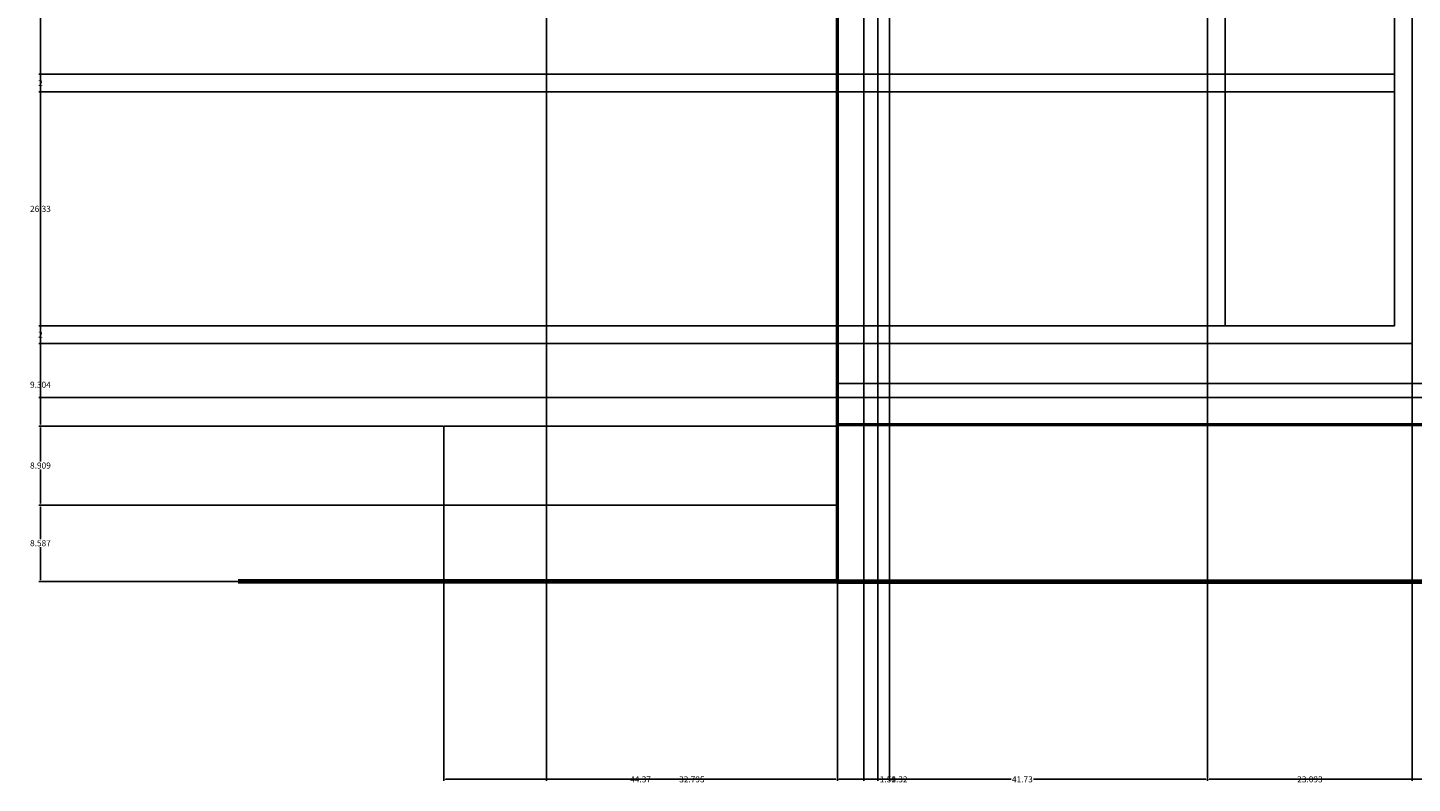
# Model space of a CAD drawing. Units: inches. Extents: x -139 to 346, y 72 to 413.
# Tile 1 of 18: x -139 to 18, y 72 to 157. Entities that reach past the tile are written whole.
import ezdxf

# ---------------------------------------------------------------- set-up
doc = ezdxf.new("R2010")
doc.units = ezdxf.units.IN
doc.header["$MEASUREMENT"] = 0
for name, color, linetype, lineweight in [('A-ANNO-DIMS', 2, 'Continuous', 18), ('A-FLOR-STRS', 2, 'Continuous', 25), ('A-GLAZ', 4, 'Continuous', 25), ('A-WALL', 7, 'Continuous', 50), ('C-TOPO', 7, 'Continuous', 70)]:
    doc.layers.add(name, color=color, linetype=linetype, lineweight=lineweight)
doc.styles.get("Standard").update_dxf_attribs({"font": 'arial.ttf'})
doc.dimstyles.get("Standard").update_dxf_attribs({"dimtxt": 0.6875, "dimasz": 0.18, "dimexe": 0.18, "dimexo": 0.0625, "dimgap": 0.09, "dimtad": 0, "dimtih": 1, "dimtoh": 1, "dimdec": 4, "dimzin": 0, "dimdsep": 46, "dimlunit": 4, "dimtxsty": 'Standard', "dimcen": 0.09, "dimadec": 0, "dimazin": 0, "dimtfac": 1, "dimtdec": 4, "dimtofl": 0, "dimtmove": 0, "dimatfit": 3, "dimfxl": 1, "dimtolj": 1, "dimtzin": 0, "dimarcsym": 0})

# ---------------------------------------------------------------- blocks, each defined once
blk = doc.blocks.new('*D7')
at = {"layer": 'A-ANNO-DIMS', "color": 0, "lineweight": -2, "transparency": 16777216}
for p, q in [((-47.27, 95.04), (-47.27, 117.45)), ((-47.09, 117.27), (129.79, 117.27)), ((309.71, 117.27), (132.82, 117.27)), ((309.89, 95.04), (309.89, 117.45))]:
    blk.add_line(p, q, dxfattribs=at)
at = {"layer": 'A-ANNO-DIMS', "color": 0, "transparency": 16777216}
for points in [[(-47.09, 117.3), (-47.09, 117.24), (-47.27, 117.27)], [(309.71, 117.3), (309.71, 117.24), (309.89, 117.27)]]:
    blk.add_solid(points, dxfattribs=at)
at = {"layer": 'Defpoints', "color": 0, "transparency": 16777216}
for p in [(309.89, 117.27), (-47.27, 94.97), (309.89, 94.97)]:
    blk.add_point(p, dxfattribs=at)
at = {"layer": 'A-ANNO-DIMS', "color": 0, "transparency": 16777216, "insert": (131.31, 117.27), "char_height": 0.688, "attachment_point": 5}
blk.add_mtext('\\A1;357.16', dxfattribs=at)
blk = doc.blocks.new('*D8')
at = {"layer": 'A-ANNO-DIMS', "color": 0, "lineweight": -2, "transparency": 16777216}
for p, q in [((-91.64, 94.91), (-91.64, 72.49)), ((-47.27, 94.91), (-47.27, 72.49)), ((-91.46, 72.67), (-70.72, 72.67)), ((-47.45, 72.67), (-68.19, 72.67))]:
    blk.add_line(p, q, dxfattribs=at)
at = {"layer": 'A-ANNO-DIMS', "color": 0, "transparency": 16777216}
for points in [[(-91.46, 72.7), (-91.46, 72.64), (-91.64, 72.67)], [(-47.45, 72.7), (-47.45, 72.64), (-47.27, 72.67)]]:
    blk.add_solid(points, dxfattribs=at)
at = {"layer": 'Defpoints', "color": 0, "transparency": 16777216}
for p in [(-91.64, 94.97), (-47.27, 94.97), (-47.27, 72.67)]:
    blk.add_point(p, dxfattribs=at)
at = {"layer": 'A-ANNO-DIMS', "color": 0, "transparency": 16777216, "insert": (-69.46, 72.67), "char_height": 0.688, "attachment_point": 5}
blk.add_mtext('\\A1;44.37', dxfattribs=at)
blk = doc.blocks.new('*D9')
at = {"layer": 'A-ANNO-DIMS', "color": 0, "lineweight": -2, "transparency": 16777216}
for p, q in [((-5.54, 121.71), (-5.54, 72.49)), ((-47.27, 112.54), (-47.27, 72.49)), ((-47.09, 72.67), (-27.67, 72.67)), ((-5.72, 72.67), (-25.14, 72.67))]:
    blk.add_line(p, q, dxfattribs=at)
at = {"layer": 'A-ANNO-DIMS', "color": 0, "transparency": 16777216}
for points in [[(-47.09, 72.7), (-47.09, 72.64), (-47.27, 72.67)], [(-5.72, 72.7), (-5.72, 72.64), (-5.54, 72.67)]]:
    blk.add_solid(points, dxfattribs=at)
at = {"layer": 'Defpoints', "color": 0, "transparency": 16777216}
for p in [(-5.54, 121.78), (-47.27, 112.6), (-5.54, 72.67)]:
    blk.add_point(p, dxfattribs=at)
at = {"layer": 'A-ANNO-DIMS', "color": 0, "transparency": 16777216, "insert": (-26.41, 72.67), "char_height": 0.688, "attachment_point": 5}
blk.add_mtext('\\A1;41.73', dxfattribs=at)
blk = doc.blocks.new('*D10')
at = {"layer": 'A-ANNO-DIMS', "color": 0, "lineweight": -2, "transparency": 16777216}
for p, q in [((-5.54, 121.71), (-5.54, 72.49)), ((112.65, 112.54), (112.65, 72.49)), ((-5.36, 72.67), (52.34, 72.67)), ((112.47, 72.67), (54.77, 72.67))]:
    blk.add_line(p, q, dxfattribs=at)
at = {"layer": 'A-ANNO-DIMS', "color": 0, "transparency": 16777216}
for points in [[(-5.36, 72.7), (-5.36, 72.64), (-5.54, 72.67)], [(112.47, 72.7), (112.47, 72.64), (112.65, 72.67)]]:
    blk.add_solid(points, dxfattribs=at)
at = {"layer": 'Defpoints', "color": 0, "transparency": 16777216}
for p in [(-5.54, 121.78), (112.65, 112.6), (112.65, 72.67)]:
    blk.add_point(p, dxfattribs=at)
at = {"layer": 'A-ANNO-DIMS', "color": 0, "transparency": 16777216, "insert": (53.56, 72.67), "char_height": 0.688, "attachment_point": 5}
blk.add_mtext('\\A1;118.2', dxfattribs=at)
blk = doc.blocks.new('*D12')
at = {"layer": 'A-ANNO-DIMS', "color": 0, "lineweight": -2, "transparency": 16777216}
for p, q in [((-5.54, 121.71), (-5.54, 72.49)), ((17.55, 121.71), (17.55, 72.49)), ((-5.36, 72.67), (4.48, 72.67)), ((17.37, 72.67), (7.53, 72.67))]:
    blk.add_line(p, q, dxfattribs=at)
at = {"layer": 'A-ANNO-DIMS', "color": 0, "transparency": 16777216}
for points in [[(-5.36, 72.7), (-5.36, 72.64), (-5.54, 72.67)], [(17.37, 72.7), (17.37, 72.64), (17.55, 72.67)]]:
    blk.add_solid(points, dxfattribs=at)
at = {"layer": 'Defpoints', "color": 0, "transparency": 16777216}
for p in [(-5.54, 121.78), (17.55, 121.78), (17.55, 72.67)]:
    blk.add_point(p, dxfattribs=at)
at = {"layer": 'A-ANNO-DIMS', "color": 0, "transparency": 16777216, "insert": (6.01, 72.67), "char_height": 0.688, "attachment_point": 5}
blk.add_mtext('\\A1;23.093', dxfattribs=at)
blk = doc.blocks.new('*D38')
at = {"layer": 'A-ANNO-DIMS', "color": 0, "lineweight": -2, "transparency": 16777216}
for p, q in [((-91.7, 103.56), (-137.3, 103.56)), ((-137.12, 103.38), (-137.12, 99.71)), ((-137.12, 95.15), (-137.12, 98.83)), ((-47.34, 94.97), (-137.3, 94.97))]:
    blk.add_line(p, q, dxfattribs=at)
at = {"layer": 'A-ANNO-DIMS', "color": 0, "transparency": 16777216}
for points in [[(-137.15, 103.38), (-137.09, 103.38), (-137.12, 103.56)], [(-137.15, 95.15), (-137.09, 95.15), (-137.12, 94.97)]]:
    blk.add_solid(points, dxfattribs=at)
at = {"layer": 'Defpoints', "color": 0, "transparency": 16777216}
for p in [(-137.12, 103.56), (-91.64, 103.56), (-47.27, 94.97)]:
    blk.add_point(p, dxfattribs=at)
at = {"layer": 'A-ANNO-DIMS', "color": 0, "transparency": 16777216, "insert": (-137.12, 99.27), "char_height": 0.688, "attachment_point": 5}
blk.add_mtext('\\A1;8.587', dxfattribs=at)
blk = doc.blocks.new('*D39')
at = {"layer": 'A-ANNO-DIMS', "color": 0, "lineweight": -2, "transparency": 16777216}
for p, q in [((-91.7, 112.47), (-137.3, 112.47)), ((-137.12, 112.29), (-137.12, 108.46)), ((-137.12, 103.74), (-137.12, 107.58)), ((-91.7, 103.56), (-137.3, 103.56))]:
    blk.add_line(p, q, dxfattribs=at)
at = {"layer": 'A-ANNO-DIMS', "color": 0, "transparency": 16777216}
for points in [[(-137.15, 112.29), (-137.09, 112.29), (-137.12, 112.47)], [(-137.15, 103.74), (-137.09, 103.74), (-137.12, 103.56)]]:
    blk.add_solid(points, dxfattribs=at)
at = {"layer": 'Defpoints', "color": 0, "transparency": 16777216}
for p in [(-137.12, 112.47), (-91.64, 112.47), (-91.64, 103.56)]:
    blk.add_point(p, dxfattribs=at)
at = {"layer": 'A-ANNO-DIMS', "color": 0, "transparency": 16777216, "insert": (-137.12, 108.02), "char_height": 0.688, "attachment_point": 5}
blk.add_mtext('\\A1;8.909', dxfattribs=at)
blk = doc.blocks.new('*D40')
at = {"layer": 'A-ANNO-DIMS', "color": 0, "lineweight": -2, "transparency": 16777216}
for p, q in [((-5.6, 121.78), (-137.3, 121.78)), ((-137.12, 121.6), (-137.12, 117.56)), ((-137.12, 112.65), (-137.12, 116.68)), ((-91.7, 112.47), (-137.3, 112.47))]:
    blk.add_line(p, q, dxfattribs=at)
at = {"layer": 'A-ANNO-DIMS', "color": 0, "transparency": 16777216}
for points in [[(-137.15, 121.6), (-137.09, 121.6), (-137.12, 121.78)], [(-137.15, 112.65), (-137.09, 112.65), (-137.12, 112.47)]]:
    blk.add_solid(points, dxfattribs=at)
at = {"layer": 'Defpoints', "color": 0, "transparency": 16777216}
for p in [(-137.12, 121.78), (-5.54, 121.78), (-91.64, 112.47)]:
    blk.add_point(p, dxfattribs=at)
at = {"layer": 'A-ANNO-DIMS', "color": 0, "transparency": 16777216, "insert": (-137.12, 117.12), "char_height": 0.688, "attachment_point": 5}
blk.add_mtext('\\A1;9.304', dxfattribs=at)
blk = doc.blocks.new('*D41')
at = {"layer": 'A-ANNO-DIMS', "color": 0, "lineweight": -2, "transparency": 16777216}
for p, q in [((-47.34, 207.52), (-137.3, 207.52)), ((-137.12, 207.34), (-137.12, 165.09)), ((-137.12, 121.96), (-137.12, 164.21)), ((-5.6, 121.78), (-137.3, 121.78))]:
    blk.add_line(p, q, dxfattribs=at)
at = {"layer": 'A-ANNO-DIMS', "color": 0, "transparency": 16777216}
for points in [[(-137.15, 207.34), (-137.09, 207.34), (-137.12, 207.52)], [(-137.15, 121.96), (-137.09, 121.96), (-137.12, 121.78)]]:
    blk.add_solid(points, dxfattribs=at)
at = {"layer": 'Defpoints', "color": 0, "transparency": 16777216}
for p in [(-137.12, 207.52), (-47.27, 207.52), (-5.54, 121.78)]:
    blk.add_point(p, dxfattribs=at)
at = {"layer": 'A-ANNO-DIMS', "color": 0, "transparency": 16777216, "insert": (-137.12, 164.65), "char_height": 0.688, "attachment_point": 5}
blk.add_mtext('\\A1;85.75', dxfattribs=at)
blk = doc.blocks.new('*D51')
at = {"layer": 'A-ANNO-DIMS', "color": 0, "lineweight": -2, "transparency": 16777216}
for p, q in [((-80.07, 207.46), (-80.07, 72.49)), ((-47.27, 207.46), (-47.27, 72.49)), ((-79.89, 72.67), (-65.19, 72.67)), ((-47.45, 72.67), (-62.15, 72.67))]:
    blk.add_line(p, q, dxfattribs=at)
at = {"layer": 'A-ANNO-DIMS', "color": 0, "transparency": 16777216}
for points in [[(-79.89, 72.7), (-79.89, 72.64), (-80.07, 72.67)], [(-47.45, 72.7), (-47.45, 72.64), (-47.27, 72.67)]]:
    blk.add_solid(points, dxfattribs=at)
at = {"layer": 'Defpoints', "color": 0, "transparency": 16777216}
for p in [(-80.07, 207.52), (-47.27, 207.52), (-47.27, 72.67)]:
    blk.add_point(p, dxfattribs=at)
at = {"layer": 'A-ANNO-DIMS', "color": 0, "transparency": 16777216, "insert": (-63.67, 72.67), "char_height": 0.688, "attachment_point": 5}
blk.add_mtext('\\A1;32.795', dxfattribs=at)
blk = doc.blocks.new('*D56')
at = {"layer": 'A-ANNO-DIMS', "color": 0, "lineweight": -2, "transparency": 16777216}
for p, q in [((-3.6, 123.78), (-137.3, 123.78)), ((-137.12, 123.6), (-137.12, 123.21)), ((-5.6, 121.78), (-137.3, 121.78)), ((-137.12, 121.96), (-137.12, 122.34))]:
    blk.add_line(p, q, dxfattribs=at)
at = {"layer": 'A-ANNO-DIMS', "color": 0, "transparency": 16777216}
for points in [[(-137.15, 123.6), (-137.09, 123.6), (-137.12, 123.78)], [(-137.15, 121.96), (-137.09, 121.96), (-137.12, 121.78)]]:
    blk.add_solid(points, dxfattribs=at)
at = {"layer": 'Defpoints', "color": 0, "transparency": 16777216}
for p in [(-137.12, 123.78), (-3.54, 123.78), (-5.54, 121.78)]:
    blk.add_point(p, dxfattribs=at)
at = {"layer": 'A-ANNO-DIMS', "color": 0, "transparency": 16777216, "insert": (-137.12, 122.78), "char_height": 0.688, "attachment_point": 5}
blk.add_mtext('\\A1;2', dxfattribs=at)
blk = doc.blocks.new('*D57')
at = {"layer": 'A-ANNO-DIMS', "color": 0, "lineweight": -2, "transparency": 16777216}
for p, q in [((-3.6, 150.11), (-137.3, 150.11)), ((-137.12, 149.93), (-137.12, 137.38)), ((-137.12, 123.96), (-137.12, 136.5)), ((-3.6, 123.78), (-137.3, 123.78))]:
    blk.add_line(p, q, dxfattribs=at)
at = {"layer": 'A-ANNO-DIMS', "color": 0, "transparency": 16777216}
for points in [[(-137.15, 149.93), (-137.09, 149.93), (-137.12, 150.11)], [(-137.15, 123.96), (-137.09, 123.96), (-137.12, 123.78)]]:
    blk.add_solid(points, dxfattribs=at)
at = {"layer": 'Defpoints', "color": 0, "transparency": 16777216}
for p in [(-137.12, 150.11), (-3.54, 150.11), (-3.54, 123.78)]:
    blk.add_point(p, dxfattribs=at)
at = {"layer": 'A-ANNO-DIMS', "color": 0, "transparency": 16777216, "insert": (-137.12, 136.94), "char_height": 0.688, "attachment_point": 5}
blk.add_mtext('\\A1;26.33', dxfattribs=at)
blk = doc.blocks.new('*D58')
at = {"layer": 'A-ANNO-DIMS', "color": 0, "lineweight": -2, "transparency": 16777216}
for p, q in [((-3.6, 152.11), (-137.3, 152.11)), ((-137.12, 151.93), (-137.12, 151.54)), ((-3.6, 150.11), (-137.3, 150.11)), ((-137.12, 150.29), (-137.12, 150.67))]:
    blk.add_line(p, q, dxfattribs=at)
at = {"layer": 'A-ANNO-DIMS', "color": 0, "transparency": 16777216}
for points in [[(-137.15, 151.93), (-137.09, 151.93), (-137.12, 152.11)], [(-137.15, 150.29), (-137.09, 150.29), (-137.12, 150.11)]]:
    blk.add_solid(points, dxfattribs=at)
at = {"layer": 'Defpoints', "color": 0, "transparency": 16777216}
for p in [(-137.12, 152.11), (-3.54, 152.11), (-3.54, 150.11)]:
    blk.add_point(p, dxfattribs=at)
at = {"layer": 'A-ANNO-DIMS', "color": 0, "transparency": 16777216, "insert": (-137.12, 151.11), "char_height": 0.688, "attachment_point": 5}
blk.add_mtext('\\A1;2', dxfattribs=at)
blk = doc.blocks.new('*D59')
at = {"layer": 'A-ANNO-DIMS', "color": 0, "lineweight": -2, "transparency": 16777216}
for p, q in [((-3.6, 205.52), (-137.3, 205.52)), ((-137.12, 205.34), (-137.12, 179.26)), ((-137.12, 152.29), (-137.12, 178.37)), ((-3.6, 152.11), (-137.3, 152.11))]:
    blk.add_line(p, q, dxfattribs=at)
at = {"layer": 'A-ANNO-DIMS', "color": 0, "transparency": 16777216}
for points in [[(-137.15, 205.34), (-137.09, 205.34), (-137.12, 205.52)], [(-137.15, 152.29), (-137.09, 152.29), (-137.12, 152.11)]]:
    blk.add_solid(points, dxfattribs=at)
at = {"layer": 'Defpoints', "color": 0, "transparency": 16777216}
for p in [(-137.12, 205.52), (-3.54, 205.52), (-3.54, 152.11)]:
    blk.add_point(p, dxfattribs=at)
at = {"layer": 'A-ANNO-DIMS', "color": 0, "transparency": 16777216, "insert": (-137.12, 178.82), "char_height": 0.688, "attachment_point": 5}
blk.add_mtext('\\A1;53.42', dxfattribs=at)
blk = doc.blocks.new('*D61')
at = {"layer": 'A-ANNO-DIMS', "color": 0, "lineweight": -2, "transparency": 16777216}
for p, q in [((-5.6, 207.52), (-137.3, 207.52)), ((-137.12, 207.34), (-137.12, 165.09)), ((-137.12, 121.96), (-137.12, 164.21)), ((-5.6, 121.78), (-137.3, 121.78))]:
    blk.add_line(p, q, dxfattribs=at)
at = {"layer": 'A-ANNO-DIMS', "color": 0, "transparency": 16777216}
for points in [[(-137.15, 207.34), (-137.09, 207.34), (-137.12, 207.52)], [(-137.15, 121.96), (-137.09, 121.96), (-137.12, 121.78)]]:
    blk.add_solid(points, dxfattribs=at)
at = {"layer": 'Defpoints', "color": 0, "transparency": 16777216}
for p in [(-137.12, 207.52), (-5.54, 207.52), (-5.54, 121.78)]:
    blk.add_point(p, dxfattribs=at)
at = {"layer": 'A-ANNO-DIMS', "color": 0, "transparency": 16777216, "insert": (-137.12, 164.65), "char_height": 0.688, "attachment_point": 5}
blk.add_mtext('\\A1;85.75', dxfattribs=at)
blk = doc.blocks.new('*D70')
at = {"layer": 'A-ANNO-DIMS', "color": 0, "lineweight": -2, "transparency": 16777216}
for p, q in [((125.18, 218.06), (-137.3, 218.06)), ((-137.12, 217.88), (-137.12, 167.31)), ((-137.12, 115.86), (-137.12, 166.43)), ((125.18, 115.68), (-137.3, 115.68))]:
    blk.add_line(p, q, dxfattribs=at)
at = {"layer": 'A-ANNO-DIMS', "color": 0, "transparency": 16777216}
for points in [[(-137.15, 217.88), (-137.09, 217.88), (-137.12, 218.06)], [(-137.15, 115.86), (-137.09, 115.86), (-137.12, 115.68)]]:
    blk.add_solid(points, dxfattribs=at)
at = {"layer": 'Defpoints', "color": 0, "transparency": 16777216}
for p in [(-137.12, 218.06), (125.25, 218.06), (125.25, 115.68)]:
    blk.add_point(p, dxfattribs=at)
at = {"layer": 'A-ANNO-DIMS', "color": 0, "transparency": 16777216, "insert": (-137.12, 166.87), "char_height": 0.688, "attachment_point": 5}
blk.add_mtext('\\A1;102.39', dxfattribs=at)
blk = doc.blocks.new('*D93')
at = {"layer": 'A-ANNO-DIMS', "color": 0, "lineweight": -2, "transparency": 16777216}
for p, q in [((-44.29, 298.23), (-44.29, 72.49)), ((-42.71, 291), (-42.71, 72.49)), ((-44.11, 72.67), (-42.89, 72.67)), ((-42.71, 72.67), (-42.53, 72.67))]:
    blk.add_line(p, q, dxfattribs=at)
at = {"layer": 'A-ANNO-DIMS', "color": 0, "transparency": 16777216}
for points in [[(-44.11, 72.7), (-44.11, 72.64), (-44.29, 72.67)], [(-42.89, 72.7), (-42.89, 72.64), (-42.71, 72.67)]]:
    blk.add_solid(points, dxfattribs=at)
at = {"layer": 'Defpoints', "color": 0, "transparency": 16777216}
for p in [(-44.29, 298.29), (-42.71, 291.06), (-42.71, 72.67)]:
    blk.add_point(p, dxfattribs=at)
at = {"layer": 'A-ANNO-DIMS', "color": 0, "transparency": 16777216, "insert": (-41.58, 72.67), "char_height": 0.688, "attachment_point": 5}
blk.add_mtext('\\A1;1.58', dxfattribs=at)
blk = doc.blocks.new('*D94')
at = {"layer": 'A-ANNO-DIMS', "color": 0, "lineweight": -2, "transparency": 16777216}
for p, q in [((-42.71, 291), (-42.71, 72.49)), ((-41.4, 291), (-41.4, 72.49)), ((-42.53, 72.67), (-41.58, 72.67)), ((-41.4, 72.67), (-41.22, 72.67))]:
    blk.add_line(p, q, dxfattribs=at)
at = {"layer": 'A-ANNO-DIMS', "color": 0, "transparency": 16777216}
for points in [[(-42.53, 72.7), (-42.53, 72.64), (-42.71, 72.67)], [(-41.58, 72.7), (-41.58, 72.64), (-41.4, 72.67)]]:
    blk.add_solid(points, dxfattribs=at)
at = {"layer": 'Defpoints', "color": 0, "transparency": 16777216}
for p in [(-42.71, 291.06), (-41.4, 291.06), (-41.4, 72.67)]:
    blk.add_point(p, dxfattribs=at)
at = {"layer": 'A-ANNO-DIMS', "color": 0, "transparency": 16777216, "insert": (-40.27, 72.67), "char_height": 0.688, "attachment_point": 5}
blk.add_mtext('\\A1;1.32', dxfattribs=at)

msp = doc.modelspace()

# ---------------------------------------------------------------- linework, layer by layer
at = {"layer": 'A-FLOR-STRS'}
for p, q in [((-47.2734, 112.4712), (-91.6418, 112.4712)), ((-91.6418, 112.4712), (-91.6418, 103.5622)), ((-47.2734, 103.5622), (-91.6418, 103.5622)), ((-91.6418, 103.5622), (-91.6418, 94.9748))]:
    msp.add_line(p, q, dxfattribs=at)
at = {"layer": 'A-GLAZ'}
for p, q in [((-3.5402, 152.1076), (15.5525, 152.1076)), ((-3.5402, 150.1076), (15.5525, 150.1076))]:
    msp.add_line(p, q, dxfattribs=at)
for points in [[(-5.5402, 207.5243), (17.5525, 207.5243), (17.5525, 121.7753), (-5.5402, 121.7753)], [(-3.5402, 205.5243), (15.5525, 205.5243), (15.5525, 123.7753), (-3.5402, 123.7753)]]:
    msp.add_lwpolyline(points, close=True, dxfattribs=at)
at = {"layer": 'A-WALL'}
for p, q in [((-47.2734, 291.0604), (-47.2734, 94.9748)), ((112.6506, 112.6042), (-47.2734, 112.6042))]:
    msp.add_line(p, q, dxfattribs=at)
at = {"layer": 'C-TOPO'}
for q in [(-114.8237, 94.9748), (51.0187, 94.9748)]:
    msp.add_line((-47.2734, 94.9748), q, dxfattribs=at)

# ---------------------------------------------------------------- dimensions: what is measured, and where the dimension line sits
at = {"layer": 'A-ANNO-DIMS'}
for base, p1, p2, override, picture, middle in [((-42.7149, 72.6748), (-44.2923, 298.293), (-42.7149, 291.0604), {"dimdec": 2, "dimlfac": 1, "dimrnd": 0, "dimzin": 0, "dimdsep": 46, "dimlunit": 2}, '*D93', (-41.5836, 72.6748)), ((-41.3972, 72.6748), (-42.7149, 291.0604), (-41.3972, 291.0604), {"dimdec": 2, "dimlfac": 1, "dimrnd": 0, "dimzin": 0, "dimdsep": 46, "dimlunit": 2}, '*D94', (-40.2702, 72.6748)), ((-47.2734, 72.6748), (-80.0684, 207.5243), (-47.2734, 207.5243), {"dimdec": 3, "dimlfac": 1, "dimrnd": 0, "dimzin": 0, "dimdsep": 46, "dimlunit": 2}, '*D51', (-63.6709, 72.6748)), ((-5.5402, 72.6748), (-47.2734, 112.6042), (-5.5402, 121.7753), {"dimdec": 2, "dimlfac": 1, "dimrnd": 0, "dimzin": 0, "dimdsep": 46, "dimlunit": 2}, '*D9', (-26.4068, 72.6748)), ((112.6506, 72.6748), (-5.5402, 121.7753), (112.6506, 112.6042), {"dimdec": 1, "dimlfac": 1, "dimrnd": 0, "dimzin": 0, "dimdsep": 46, "dimlunit": 2}, '*D10', (53.5552, 72.6748)), ((17.5525, 72.6748), (-5.5402, 121.7753), (17.5525, 121.7753), {"dimdec": 3, "dimlfac": 1, "dimrnd": 0, "dimzin": 0, "dimdsep": 46, "dimlunit": 2}, '*D12', (6.0062, 72.6748)), ((309.8894, 117.2748), (-47.2734, 94.9748), (309.8894, 94.9748), {"dimdec": 2, "dimlfac": 1, "dimrnd": 0, "dimzin": 0, "dimdsep": 46, "dimlunit": 2}, '*D7', (131.308, 117.2748)), ((-47.2734, 72.6748), (-91.6418, 94.9748), (-47.2734, 94.9748), {"dimdec": 2, "dimlfac": 1, "dimrnd": 0, "dimzin": 0, "dimdsep": 46, "dimlunit": 2}, '*D8', (-69.4576, 72.6748))]:
    dim = msp.add_linear_dim(base=base, p1=p1, p2=p2, dimstyle='Standard', override=override, dxfattribs=at)
    dim.commit()
    dim.dimension.update_dxf_attribs({"geometry": picture, "text_midpoint": middle})
for base, p1, p2, override, picture, middle in [((-137.1237, 218.0635), (125.2464, 115.6761), (125.2464, 218.0635), {"dimdec": 2, "dimlfac": 1, "dimrnd": 0, "dimzin": 0, "dimdsep": 46, "dimlunit": 2}, '*D70', (-137.1237, 166.8698)), ((-137.1237, 207.5243), (-5.5402, 121.7753), (-47.2734, 207.5243), {"dimdec": 2, "dimlfac": 1, "dimrnd": 0, "dimzin": 0, "dimdsep": 46, "dimlunit": 2}, '*D41', (-137.1237, 164.6498)), ((-137.1237, 207.5243), (-5.5402, 121.7753), (-5.5402, 207.5243), {"dimdec": 2, "dimlfac": 1, "dimrnd": 0, "dimzin": 0, "dimdsep": 46, "dimlunit": 2}, '*D61', (-137.1237, 164.6498)), ((-137.1237, 205.5243), (-3.5402, 152.1076), (-3.5402, 205.5243), {"dimdec": 2, "dimlfac": 1, "dimrnd": 0, "dimzin": 0, "dimdsep": 46, "dimlunit": 2}, '*D59', (-137.1237, 178.8159)), ((-137.1237, 152.1076), (-3.5402, 150.1076), (-3.5402, 152.1076), {"dimdec": 0, "dimlfac": 1, "dimrnd": 0, "dimzin": 0, "dimdsep": 46, "dimlunit": 2}, '*D58', (-137.1237, 151.1076)), ((-137.1237, 150.1076), (-3.5402, 123.7753), (-3.5402, 150.1076), {"dimdec": 2, "dimlfac": 1, "dimrnd": 0, "dimzin": 0, "dimdsep": 46, "dimlunit": 2}, '*D57', (-137.1237, 136.9414)), ((-137.1237, 123.7753), (-5.5402, 121.7753), (-3.5402, 123.7753), {"dimdec": 0, "dimlfac": 1, "dimrnd": 0, "dimzin": 0, "dimdsep": 46, "dimlunit": 2}, '*D56', (-137.1237, 122.7753)), ((-137.1237, 121.7753), (-91.6418, 112.4712), (-5.5402, 121.7753), {"dimdec": 3, "dimlfac": 1, "dimrnd": 0, "dimzin": 0, "dimdsep": 46, "dimlunit": 2}, '*D40', (-137.1237, 117.1232)), ((-137.1237, 112.4712), (-91.6418, 103.5622), (-91.6418, 112.4712), {"dimdec": 3, "dimlfac": 1, "dimrnd": 0, "dimzin": 0, "dimdsep": 46, "dimlunit": 2}, '*D39', (-137.1237, 108.0167)), ((-137.1237, 103.5622), (-47.2734, 94.9748), (-91.6418, 103.5622), {"dimdec": 3, "dimlfac": 1, "dimrnd": 0, "dimzin": 0, "dimdsep": 46, "dimlunit": 2}, '*D38', (-137.1237, 99.2685))]:
    dim = msp.add_linear_dim(base=base, p1=p1, p2=p2, angle=90, dimstyle='Standard', override=override, dxfattribs=at)
    dim.commit()
    dim.dimension.update_dxf_attribs({"geometry": picture, "text_midpoint": middle})

doc.saveas('drawing.dxf')
